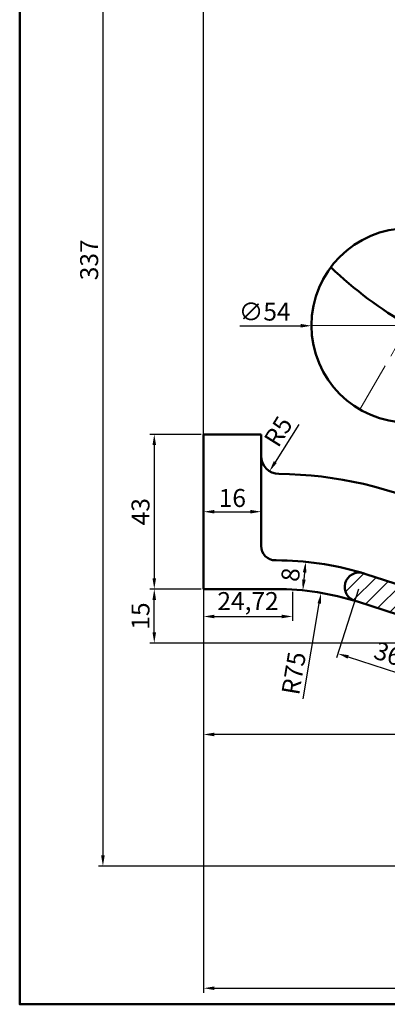
# Model space of a CAD drawing. Units: millimetres. Extents: x 98 to 674, y 38 to 476.
# Tile 1 of 7: x 98 to 200, y 38 to 312. Entities that reach past the tile are written whole.
import ezdxf

# ---------------------------------------------------------------- set-up
doc = ezdxf.new("R2010")
doc.units = ezdxf.units.MM
doc.header["$LTSCALE"] = 0.5
doc.linetypes.add('CENTER', pattern=[50.8, 31.75, -6.35, 6.35, -6.35])
for name, color, linetype, lineweight in [('M-CNTR', 1, 'CENTER', 18), ('M-DIMS', 2, 'Continuous', 25), ('M-HATC', 8, 'Continuous', 18), ('M-OUTL', 7, 'Continuous', 50), ('M-TTLB', 7, 'Continuous', 50)]:
    doc.layers.add(name, color=color, linetype=linetype, lineweight=lineweight)
doc.styles.get("Standard").update_dxf_attribs({"font": 'arial.ttf'})
doc.dimstyles.new('ISO-25', dxfattribs={"dimtxt": 5, "dimasz": 3, "dimexe": 1.25, "dimexo": 0.625, "dimtad": 1, "dimtxsty": 'Standard', "dimcen": 2.5, "dimadec": 0, "dimazin": 0, "dimtfac": 1, "dimtmove": 0, "dimatfit": 3, "dimfxl": 1, "dimarcsym": 0})

# ---------------------------------------------------------------- blocks, each defined once
blk = doc.blocks.new('*D50')
at = {"layer": 'Defpoints', "color": 0, "ltscale": 0.5, "transparency": 16777216}
for p in [(149.37, 153.69), (149.37, 113.28), (277.37, 112.69)]:
    blk.add_point(p, dxfattribs=at)
at = {"layer": 'M-DIMS', "color": 0, "lineweight": -2, "ltscale": 0.5, "transparency": 16777216}
for p, q in [((149.37, 153.06), (149.37, 112.03)), ((274.37, 113.28), (152.37, 113.28)), ((277.37, 113.31), (277.37, 114.53))]:
    blk.add_line(p, q, dxfattribs=at)
at = {"layer": 'M-DIMS', "color": 0, "ltscale": 0.5, "transparency": 16777216}
for points in [[(152.37, 113.78), (152.37, 112.78), (149.37, 113.28)], [(274.37, 113.78), (274.37, 112.78), (277.37, 113.28)]]:
    blk.add_solid(points, dxfattribs=at)
at = {"layer": 'M-DIMS', "color": 0, "ltscale": 0.5, "transparency": 16777216, "insert": (213.37, 116.46), "char_height": 5, "attachment_point": 5}
blk.add_mtext('128', dxfattribs=at)
blk = doc.blocks.new('*D51')
at = {"layer": 'Defpoints', "color": 0, "ltscale": 0.5, "transparency": 16777216}
for p in [(149.37, 196.69), (135.65, 153.69), (149.37, 153.69)]:
    blk.add_point(p, dxfattribs=at)
at = {"layer": 'M-DIMS', "color": 0, "lineweight": -2, "ltscale": 0.5, "transparency": 16777216}
for p, q in [((148.74, 196.69), (134.4, 196.69)), ((135.65, 193.69), (135.65, 156.69)), ((148.74, 153.69), (134.4, 153.69))]:
    blk.add_line(p, q, dxfattribs=at)
at = {"layer": 'M-DIMS', "color": 0, "ltscale": 0.5, "transparency": 16777216}
for points in [[(135.15, 193.69), (136.15, 193.69), (135.65, 196.69)], [(135.15, 156.69), (136.15, 156.69), (135.65, 153.69)]]:
    blk.add_solid(points, dxfattribs=at)
at = {"layer": 'M-DIMS', "color": 0, "ltscale": 0.5, "transparency": 16777216, "insert": (132.47, 175.19), "char_height": 5, "attachment_point": 5, "rotation": 90}
blk.add_mtext('43', dxfattribs=at)
blk = doc.blocks.new('*D52')
at = {"layer": 'Defpoints', "color": 0, "ltscale": 0.5, "transparency": 16777216}
for p in [(135.65, 153.69), (149.37, 153.69), (251.25, 138.69)]:
    blk.add_point(p, dxfattribs=at)
at = {"layer": 'M-DIMS', "color": 0, "lineweight": -2, "ltscale": 0.5, "transparency": 16777216}
for p, q in [((148.74, 153.69), (134.4, 153.69)), ((135.65, 141.69), (135.65, 150.69)), ((250.63, 138.69), (134.4, 138.69))]:
    blk.add_line(p, q, dxfattribs=at)
at = {"layer": 'M-DIMS', "color": 0, "ltscale": 0.5, "transparency": 16777216}
for points in [[(135.15, 150.69), (136.15, 150.69), (135.65, 153.69)], [(135.15, 141.69), (136.15, 141.69), (135.65, 138.69)]]:
    blk.add_solid(points, dxfattribs=at)
at = {"layer": 'M-DIMS', "color": 0, "ltscale": 0.5, "transparency": 16777216, "insert": (132.47, 146.19), "char_height": 5, "attachment_point": 5, "rotation": 90}
blk.add_mtext('15', dxfattribs=at)
blk = doc.blocks.new('*D53')
at = {"layer": 'Defpoints', "color": 0, "ltscale": 0.5, "transparency": 16777216}
for p in [(192.69, 154.23), (227.02, 143.17), (221.06, 124.69)]:
    blk.add_point(p, dxfattribs=at)
at = {"layer": 'M-DIMS', "color": 0, "lineweight": -2, "ltscale": 0.5, "transparency": 16777216}
for p, q in [((192.5, 153.64), (186.35, 134.56)), ((226.82, 142.58), (220.68, 123.5)), ((189.59, 134.83), (218.21, 125.61))]:
    blk.add_line(p, q, dxfattribs=at)
at = {"layer": 'M-DIMS', "color": 0, "ltscale": 0.5, "transparency": 16777216}
for points in [[(189.75, 135.31), (189.44, 134.36), (186.74, 135.75)], [(218.36, 126.09), (218.05, 125.14), (221.06, 124.69)]]:
    blk.add_solid(points, dxfattribs=at)
at = {"layer": 'M-DIMS', "color": 0, "ltscale": 0.5, "transparency": 16777216, "insert": (205.01, 133.68), "char_height": 5, "attachment_point": 5, "rotation": 342.137}
blk.add_mtext('36,06', dxfattribs=at)
blk = doc.blocks.new('*D55')
at = {"layer": 'Defpoints', "color": 0, "ltscale": 0.5, "transparency": 16777216}
for p in [(177.76, 161.28), (176.97, 153.32), (176.97, 153.32)]:
    blk.add_point(p, dxfattribs=at)
at = {"layer": 'M-DIMS', "color": 0, "lineweight": -2, "ltscale": 0.5, "transparency": 16777216}
for p, q in [((177.14, 161.35), (176.51, 161.41)), ((177.46, 158.3), (177.27, 156.31)), ((176.35, 153.38), (175.73, 153.45))]:
    blk.add_line(p, q, dxfattribs=at)
at = {"layer": 'M-DIMS', "color": 0, "ltscale": 0.5, "transparency": 16777216}
for points in [[(176.97, 158.35), (177.96, 158.25), (177.76, 161.28)], [(176.77, 156.36), (177.76, 156.26), (176.97, 153.32)]]:
    blk.add_solid(points, dxfattribs=at)
at = {"layer": 'M-DIMS', "color": 0, "ltscale": 0.5, "transparency": 16777216, "insert": (174.2, 157.62), "char_height": 5, "attachment_point": 5, "rotation": 84.3598}
blk.add_mtext('8', dxfattribs=at)
blk = doc.blocks.new('*D56')
at = {"layer": 'Defpoints', "color": 0, "ltscale": 0.5, "transparency": 16777216}
for p in [(170.37, 190.68), (167.72, 186.44)]:
    blk.add_point(p, dxfattribs=at)
at = {"layer": 'M-DIMS', "color": 0, "lineweight": -2, "ltscale": 0.5, "transparency": 16777216}
blk.add_line((175.84, 199.47), (169.31, 188.99), dxfattribs=at)
at = {"layer": 'M-DIMS', "color": 0, "ltscale": 0.5, "transparency": 16777216}
blk.add_solid([(168.88, 189.25), (169.73, 188.72), (167.72, 186.44)], dxfattribs=at)
at = {"layer": 'M-DIMS', "color": 0, "ltscale": 0.5, "transparency": 16777216, "insert": (170.68, 197.17), "char_height": 5, "attachment_point": 5, "rotation": 58.0912}
blk.add_mtext('R5', dxfattribs=at)
blk = doc.blocks.new('*D57')
at = {"layer": 'Defpoints', "color": 0, "ltscale": 0.5, "transparency": 16777216}
for p in [(149.37, 175.19), (165.37, 175.19), (165.37, 175.19)]:
    blk.add_point(p, dxfattribs=at)
at = {"layer": 'M-DIMS', "color": 0, "lineweight": -2, "ltscale": 0.5, "transparency": 16777216}
for p, q in [((149.37, 175.81), (149.37, 176.44)), ((152.37, 175.19), (162.37, 175.19)), ((165.37, 175.81), (165.37, 176.44))]:
    blk.add_line(p, q, dxfattribs=at)
at = {"layer": 'M-DIMS', "color": 0, "ltscale": 0.5, "transparency": 16777216}
for points in [[(152.37, 175.69), (152.37, 174.69), (149.37, 175.19)], [(162.37, 175.69), (162.37, 174.69), (165.37, 175.19)]]:
    blk.add_solid(points, dxfattribs=at)
at = {"layer": 'M-DIMS', "color": 0, "ltscale": 0.5, "transparency": 16777216, "insert": (157.37, 178.36), "char_height": 5, "attachment_point": 5}
blk.add_mtext('16', dxfattribs=at)
blk = doc.blocks.new('*D58')
at = {"layer": 'Defpoints', "color": 0, "ltscale": 0.5, "transparency": 16777216}
for p in [(149.37, 153.69), (174.09, 153.55), (174.09, 146.07)]:
    blk.add_point(p, dxfattribs=at)
at = {"layer": 'M-DIMS', "color": 0, "lineweight": -2, "ltscale": 0.5, "transparency": 16777216}
for p, q in [((149.37, 153.06), (149.37, 144.82)), ((174.09, 152.93), (174.09, 144.82)), ((152.37, 146.07), (171.09, 146.07))]:
    blk.add_line(p, q, dxfattribs=at)
at = {"layer": 'M-DIMS', "color": 0, "ltscale": 0.5, "transparency": 16777216}
for points in [[(152.37, 146.57), (152.37, 145.57), (149.37, 146.07)], [(171.09, 146.57), (171.09, 145.57), (174.09, 146.07)]]:
    blk.add_solid(points, dxfattribs=at)
at = {"layer": 'M-DIMS', "color": 0, "ltscale": 0.5, "transparency": 16777216, "insert": (161.73, 149.7), "char_height": 5, "attachment_point": 5}
blk.add_mtext('24,72', dxfattribs=at)
blk = doc.blocks.new('*D59')
at = {"layer": 'Defpoints', "color": 0, "ltscale": 0.5, "transparency": 16777216}
for p in [(182.06, 152.64), (169.6, 78.69)]:
    blk.add_point(p, dxfattribs=at)
at = {"layer": 'M-DIMS', "color": 0, "lineweight": -2, "ltscale": 0.5, "transparency": 16777216}
blk.add_line((177.09, 123.14), (181.56, 149.68), dxfattribs=at)
at = {"layer": 'M-DIMS', "color": 0, "ltscale": 0.5, "transparency": 16777216}
blk.add_solid([(181.07, 149.77), (182.06, 149.6), (182.06, 152.64)], dxfattribs=at)
at = {"layer": 'M-DIMS', "color": 0, "ltscale": 0.5, "transparency": 16777216, "insert": (175.07, 130.19), "char_height": 5, "attachment_point": 5, "rotation": 80.4366}
blk.add_mtext('R75', dxfattribs=at)
blk = doc.blocks.new('*D60')
at = {"layer": 'Defpoints', "color": 0, "ltscale": 0.5, "transparency": 16777216}
for p in [(179.37, 226.88), (233.36, 227.04)]:
    blk.add_point(p, dxfattribs=at)
at = {"layer": 'M-DIMS', "color": 0, "lineweight": -2, "ltscale": 0.5, "transparency": 16777216}
for p, q in [((159.46, 226.81), (176.37, 226.87)), ((233.36, 227.04), (179.37, 226.88)), ((236.36, 227.05), (239.36, 227.06))]:
    blk.add_line(p, q, dxfattribs=at)
at = {"layer": 'M-DIMS', "color": 0, "ltscale": 0.5, "transparency": 16777216}
for points in [[(176.36, 227.37), (176.37, 226.37), (179.37, 226.88)], [(236.36, 227.55), (236.37, 226.55), (233.36, 227.04)]]:
    blk.add_solid(points, dxfattribs=at)
at = {"layer": 'M-DIMS', "color": 0, "ltscale": 0.5, "transparency": 16777216, "insert": (166.36, 230.15), "char_height": 5, "attachment_point": 5, "rotation": 0.1768}
blk.add_mtext('∅54', dxfattribs=at)
blk = doc.blocks.new('BALL')
blk.add_circle((27, 27), 27)
blk.add_arc((84, 125.73), 114, 226.398, 253.602)
blk = doc.blocks.new('*D71')
at = {"layer": 'Defpoints', "color": 0, "ltscale": 0.5, "transparency": 16777216}
for p in [(269.37, 413.69), (121.37, 76.69), (269.37, 76.69)]:
    blk.add_point(p, dxfattribs=at)
at = {"layer": 'M-DIMS', "color": 0, "lineweight": -2, "ltscale": 0.5, "transparency": 16777216}
for p, q in [((268.74, 413.69), (120.12, 413.69)), ((121.37, 410.69), (121.37, 79.69)), ((268.74, 76.69), (120.12, 76.69))]:
    blk.add_line(p, q, dxfattribs=at)
at = {"layer": 'M-DIMS', "color": 0, "ltscale": 0.5, "transparency": 16777216}
for points in [[(120.87, 410.69), (121.87, 410.69), (121.37, 413.69)], [(120.87, 79.69), (121.87, 79.69), (121.37, 76.69)]]:
    blk.add_solid(points, dxfattribs=at)
at = {"layer": 'M-DIMS', "color": 0, "ltscale": 0.5, "transparency": 16777216, "insert": (118.19, 245.19), "char_height": 5, "attachment_point": 5, "rotation": 90}
blk.add_mtext('337', dxfattribs=at)
blk = doc.blocks.new('*D72')
at = {"layer": 'Defpoints', "color": 0, "ltscale": 0.5, "transparency": 16777216}
for p in [(149.37, 196.69), (323.37, 130.19), (323.37, 42.76)]:
    blk.add_point(p, dxfattribs=at)
at = {"layer": 'M-DIMS', "color": 0, "lineweight": -2, "ltscale": 0.5, "transparency": 16777216}
for p, q in [((149.37, 196.06), (149.37, 41.51)), ((323.37, 129.56), (323.37, 41.51)), ((152.37, 42.76), (320.37, 42.76))]:
    blk.add_line(p, q, dxfattribs=at)
at = {"layer": 'M-DIMS', "color": 0, "ltscale": 0.5, "transparency": 16777216}
for points in [[(152.37, 43.26), (152.37, 42.26), (149.37, 42.76)], [(320.37, 43.26), (320.37, 42.26), (323.37, 42.76)]]:
    blk.add_solid(points, dxfattribs=at)
at = {"layer": 'M-DIMS', "color": 0, "ltscale": 0.5, "transparency": 16777216, "insert": (236.37, 45.9), "char_height": 5, "attachment_point": 5}
blk.add_mtext('174', dxfattribs=at)
blk = doc.blocks.new('*D73')
at = {"layer": 'Defpoints', "color": 0, "ltscale": 0.5, "transparency": 16777216}
for p in [(221.4, 441.69), (221.4, 168.51), (149.37, 153.69)]:
    blk.add_point(p, dxfattribs=at)
at = {"layer": 'M-DIMS', "color": 0, "lineweight": -2, "ltscale": 0.5, "transparency": 16777216}
for p, q in [((149.37, 154.31), (149.37, 442.94)), ((152.37, 441.69), (218.4, 441.69)), ((221.4, 169.14), (221.4, 442.94))]:
    blk.add_line(p, q, dxfattribs=at)
at = {"layer": 'M-DIMS', "color": 0, "ltscale": 0.5, "transparency": 16777216}
for points in [[(152.37, 442.19), (152.37, 441.19), (149.37, 441.69)], [(218.4, 442.19), (218.4, 441.19), (221.4, 441.69)]]:
    blk.add_solid(points, dxfattribs=at)
at = {"layer": 'M-DIMS', "color": 0, "ltscale": 0.5, "transparency": 16777216, "insert": (185.38, 444.87), "char_height": 5, "attachment_point": 5}
blk.add_mtext('72.03', dxfattribs=at)

msp = doc.modelspace()

# ---------------------------------------------------------------- hatches: boundary and pattern name
at = {"layer": 'M-HATC', "ltscale": 0.5}
h = msp.add_hatch(dxfattribs=at)
h.set_pattern_fill('ANSI31', color=256)
h.paths.add_polyline_path([(215.3645, 153.2734), (221.3997, 168.5142, 1), (213.9617, 171.4596), (207.6565, 155.5371, -0.39645231), (205.1754, 154.3725), (194.5293, 157.8537, 1), (190.8572, 150.6104, -0.00464805), (192.1907, 150.2028), (225.763, 139.3083, 1.17062936), (227.0163, 147.2309), (216.6024, 150.6361, -0.43220072)])

# ---------------------------------------------------------------- linework, layer by layer
at = {"layer": 'M-CNTR'}
msp.add_line((263.365, 325.6855), (192.865, 203.5759), dxfattribs=at)
at = {"layer": 'M-OUTL', "ltscale": 0.5}
for p, q in [((149.365, 153.6855), (149.365, 196.6855)), ((149.365, 196.6855), (165.365, 196.6855)), ((165.365, 190.6829), (165.365, 165.6855)), ((169.6014, 161.6855), (169.365, 161.6855)), ((194.5293, 157.8537), (205.1754, 154.3725)), ((149.365, 153.6855), (169.6014, 153.6855)), ((192.1907, 150.2028), (225.763, 139.3083))]:
    msp.add_line(p, q, dxfattribs=at)
at = {"layer": 'M-OUTL'}
msp.add_lwpolyline([(259.365, 174.6855), (259.365, 174.6855, -0.41421356), (255.365, 170.6855), (234.9849, 170.6855, -0.11323701), (216.2416, 174.9855, 0.11151094), (170.3309, 185.683, -0.41221797), (165.365, 190.6829), (165.365, 196.6855)], format="xyb", dxfattribs=at)
at = {"layer": 'M-OUTL', "ltscale": 0.5}
for centre, radius, start, end in [((169.365, 165.6855), 4, 180, 270), ((192.6933, 154.232), 4.0605, 63.116651, 243.116651)]:
    msp.add_arc(centre, radius, start, end, dxfattribs=at)
at = {"layer": 'M-OUTL'}
for radius, start in [(83, 73.484775), (75, 72.470867)]:
    msp.add_arc((169.6014, 78.6855), radius, start, 90, dxfattribs=at)
at = {"layer": 'M-TTLB', "ltscale": 0.5}
msp.add_lwpolyline([(98.2162, 475.6271), (666.7064, 475.6271), (666.7064, 38.2873), (98.2162, 38.2873)], close=True, dxfattribs=at)

# ---------------------------------------------------------------- block references
at = {"layer": 'M-OUTL'}
msp.add_blockref('BALL', (179.365, 199.959), dxfattribs=at)

# ---------------------------------------------------------------- dimensions: what is measured, and where the dimension line sits
at = {"layer": 'M-DIMS', "ltscale": 0.5}
for base, p1, p2, override, picture, middle in [((221.3997, 441.6855), (149.365, 153.6855), (221.3997, 168.5142), {"dimdec": 2, "dimlfac": 1, "dimrnd": 0, "dimzin": 0, "dimdsep": 46, "dimlunit": 2}, '*D73', (185.3824, 444.8651)), ((323.365, 42.7639), (149.365, 196.6855), (323.365, 130.1855), {"dimdec": 0, "dimlfac": 1, "dimrnd": 0, "dimzin": 0, "dimdsep": 46, "dimlunit": 2}, '*D72', (236.365, 45.8992)), ((165.365, 175.1855), (149.365, 175.1855), (165.365, 175.1855), {"dimclrd": 0, "dimclre": 0, "dimclrt": 0}, '*D57', (157.365, 178.3633)), ((149.365, 113.2817), (277.365, 112.6855), (149.365, 153.6855), {"dimclrd": 0, "dimclre": 0, "dimclrt": 0}, '*D50', (213.365, 116.4596)), ((174.0876, 146.0719), (149.365, 153.6855), (174.0876, 153.5512), {"dimclrd": 0, "dimclre": 0, "dimclrt": 0}, '*D58', (161.7263, 149.7017))]:
    dim = msp.add_linear_dim(base=base, p1=p1, p2=p2, dimstyle='ISO-25', override=override, dxfattribs=at)
    dim.commit()
    dim.dimension.update_dxf_attribs({"geometry": picture, "text_midpoint": middle})
for base, p1, p2, override, picture, middle in [((121.365, 76.6855), (269.365, 413.6855), (269.365, 76.6855), {"dimdec": 0, "dimlfac": 1, "dimrnd": 0, "dimzin": 0, "dimdsep": 46, "dimlunit": 2}, '*D71', (118.1855, 245.1855)), ((135.6524, 153.6855), (149.365, 196.6855), (149.365, 153.6855), {"dimclrd": 0, "dimclre": 0, "dimclrt": 0}, '*D51', (132.4728, 175.1855)), ((135.6524, 153.6855), (251.2525, 138.6855), (149.365, 153.6855), {"dimclrd": 0, "dimclre": 0, "dimclrt": 0}, '*D52', (132.4745, 146.1855))]:
    dim = msp.add_linear_dim(base=base, p1=p1, p2=p2, angle=90, dimstyle='ISO-25', override=override, dxfattribs=at)
    dim.commit()
    dim.dimension.update_dxf_attribs({"geometry": picture, "text_midpoint": middle})
dim = msp.add_diameter_dim_2p(p1=(233.3649, 227.0419), p2=(179.3652, 226.8753), dimstyle='ISO-25', override={"dimclrd": 0, "dimclre": 0, "dimclrt": 0}, dxfattribs=at)
dim.commit()
dim.dimension.update_dxf_attribs({"geometry": '*D60', "text_midpoint": (166.3749, 226.8352), "dimtype": 163})
for center, mpoint, picture, middle in [((170.365, 190.6829), (167.7222, 186.4384), '*D56', (173.3647, 195.5005)), ((169.6014, 78.6855), (182.0618, 152.6432), '*D59', (178.1902, 129.6634))]:
    dim = msp.add_radius_dim(center=center, mpoint=mpoint, dimstyle='ISO-25', override={"dimclrd": 0, "dimclre": 0, "dimclrt": 0}, dxfattribs=at)
    dim.commit()
    dim.dimension.update_dxf_attribs({"geometry": picture, "text_midpoint": middle, "dimtype": 164})
for p1, p2, distance, picture, middle in [((177.7588, 161.2836), (176.9725, 153.3224), 0, '*D55', (174.2032, 157.6153)), ((192.6933, 154.232), (227.0163, 143.1705), -19.4157, '*D53', (205.0126, 133.6763))]:
    dim = msp.add_aligned_dim(p1=p1, p2=p2, distance=distance, dimstyle='ISO-25', override={"dimclrd": 0, "dimclre": 0, "dimclrt": 0}, dxfattribs=at)
    dim.commit()
    dim.dimension.update_dxf_attribs({"geometry": picture, "text_midpoint": middle})

doc.saveas('drawing.dxf')
